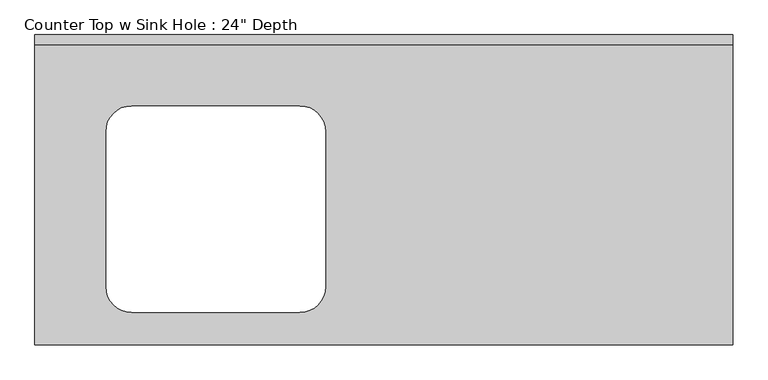
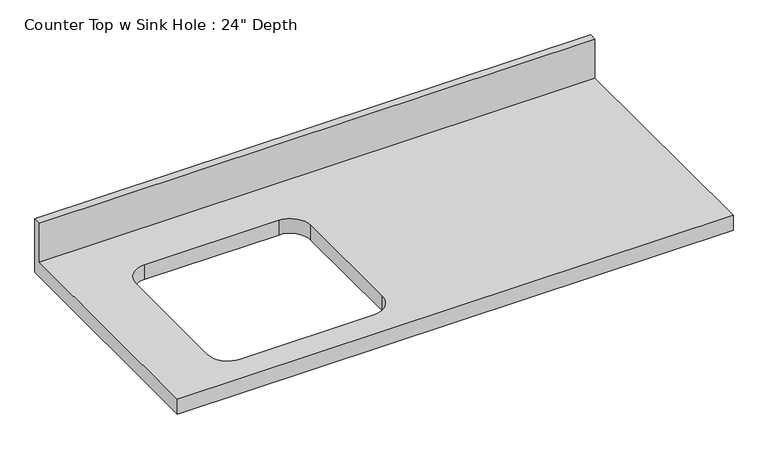
"""IFC4 building model written with IfcOpenShell, lengths in millimetres: furniture geometry."""

from ifc_helpers import new_model, si_unit, frame, origin, place, context, project, spatial, polyline, circle_curve, source, transform, mapped, element, save
from ifc_brep_helpers import plane_surface, revolved_surface, advanced_brep


def furniture_95afb093(model_context):
    return source(origin(), model_context, "Body", "AdvancedBrep", [
        advanced_brep(
        [(-1200.4622951, -609.6, 914.4), (171.1377049, -609.6, 914.4), (171.1377049, -19.05, 914.4), (-1200.4622951, -19.05, 914.4), (-1009.9622951, -139.7, 914.4), (-679.7622951, -139.7, 914.4), (-628.9622951, -190.5, 914.4), (-628.9622951, -495.3, 914.4), (-679.7622951, -546.1, 914.4), (-1009.9622951, -546.1, 914.4), (-1060.7622951, -495.3, 914.4), (-1060.7622951, -190.5, 914.4), (171.1377049, 0.0, 876.3), (171.1377049, -609.6, 876.3), (-1200.4622951, -609.6, 876.3), (-1200.4622951, 0.0, 876.3), (-679.7622951, -139.7, 876.3), (-1009.9622951, -139.7, 876.3), (-1060.7622951, -190.5, 876.3), (-1060.7622951, -495.3, 876.3), (-1009.9622951, -546.1, 876.3), (-679.7622951, -546.1, 876.3), (-628.9622951, -495.3, 876.3), (-628.9622951, -190.5, 876.3), (-1200.4622951, 0.0, 1016.0), (171.1377049, 0.0, 1016.0), (-1200.4622951, -19.05, 1016.0), (171.1377049, -19.05, 1016.0)],
        [
            (0, 1),
            (1, 2),
            (2, 3),
            (3, 0),
            (4, 5),
            (5, 6, circle_curve(frame((-679.7622951, -190.5, 914.4), z_axis=(0.0, 0.0, -1.0), x_axis=(1.0, 0.0, 0.0)), 50.8)),
            (6, 7),
            (7, 8, circle_curve(frame((-679.7622951, -495.3, 914.4), z_axis=(0.0, 0.0, -1.0), x_axis=(1.0, 0.0, 0.0)), 50.8)),
            (8, 9),
            (9, 10, circle_curve(frame((-1009.9622951, -495.3, 914.4), z_axis=(0.0, 0.0, -1.0), x_axis=(1.0, 0.0, 0.0)), 50.8)),
            (10, 11),
            (11, 4, circle_curve(frame((-1009.9622951, -190.5, 914.4), z_axis=(0.0, 0.0, -1.0), x_axis=(1.0, 0.0, 0.0)), 50.8)),
            (12, 13),
            (13, 14),
            (14, 15),
            (15, 12),
            (16, 17),
            (17, 18, circle_curve(frame((-1009.9622951, -190.5, 876.3), z_axis=(0.0, 0.0, 1.0), x_axis=(1.0, 0.0, 0.0)), 50.8)),
            (18, 19),
            (19, 20, circle_curve(frame((-1009.9622951, -495.3, 876.3), z_axis=(0.0, 0.0, 1.0), x_axis=(1.0, 0.0, 0.0)), 50.8)),
            (20, 21),
            (21, 22, circle_curve(frame((-679.7622951, -495.3, 876.3), z_axis=(0.0, 0.0, 1.0), x_axis=(1.0, 0.0, 0.0)), 50.8)),
            (22, 23),
            (23, 16, circle_curve(frame((-679.7622951, -190.5, 876.3), z_axis=(0.0, 0.0, 1.0), x_axis=(1.0, 0.0, 0.0)), 50.8)),
            (15, 24),
            (24, 25),
            (25, 12),
            (14, 0),
            (3, 26),
            (26, 24),
            (13, 1),
            (25, 27),
            (27, 2),
            (4, 17),
            (16, 5),
            (11, 18),
            (10, 19),
            (9, 20),
            (8, 21),
            (7, 22),
            (6, 23),
            (26, 27),
        ],
        [
            plane_surface(frame((-1200.4622951, 0.0, 914.4), z_axis=(0.0, 0.0, 1.0), x_axis=(-1.0, 0.0, 0.0))),
            plane_surface(frame((-1200.4622951, 0.0, 876.3), z_axis=(0.0, 0.0, -1.0), x_axis=(1.0, 0.0, 0.0))),
            plane_surface(frame((171.1377049, 0.0, 914.4), z_axis=(0.0, 1.0, 0.0), x_axis=(0.0, 0.0, -1.0))),
            plane_surface(frame((-1200.4622951, 0.0, 914.4), z_axis=(-1.0, 0.0, 0.0), x_axis=(0.0, 0.0, -1.0))),
            plane_surface(frame((-1200.4622951, -609.6, 914.4), z_axis=(0.0, -1.0, 0.0), x_axis=(0.0, 0.0, -1.0))),
            plane_surface(frame((171.1377049, -609.6, 914.4), z_axis=(1.0, 0.0, 0.0), x_axis=(0.0, 0.0, -1.0))),
            plane_surface(frame((-679.7622951, -139.7, 914.4), z_axis=(0.0, -1.0, 0.0), x_axis=(0.0, 0.0, -1.0))),
            revolved_surface(polyline([(-959.1622951, -190.5, 914.4), (-959.1622951, -190.5, 876.3)]), (-1009.9622951, -190.5, 876.3), (0.0, 0.0, 1.0)),
            plane_surface(frame((-1060.7622951, -190.5, 914.4), z_axis=(1.0, 0.0, 0.0), x_axis=(0.0, 0.0, -1.0))),
            revolved_surface(polyline([(-959.1622951, -495.3, 914.4), (-959.1622951, -495.3, 876.3)]), (-1009.9622951, -495.3, 876.3), (0.0, 0.0, 1.0)),
            plane_surface(frame((-1009.9622951, -546.1, 914.4), z_axis=(0.0, 1.0, 0.0), x_axis=(0.0, 0.0, -1.0))),
            revolved_surface(polyline([(-628.9622951, -495.3, 914.4), (-628.9622951, -495.3, 876.3)]), (-679.7622951, -495.3, 876.3), (0.0, 0.0, 1.0)),
            plane_surface(frame((-628.9622951, -495.3, 914.4), z_axis=(-1.0, 0.0, 0.0), x_axis=(0.0, 0.0, -1.0))),
            revolved_surface(polyline([(-628.9622951, -190.5, 914.4), (-628.9622951, -190.5, 876.3)]), (-679.7622951, -190.5, 876.3), (0.0, 0.0, 1.0)),
            plane_surface(frame((-1200.4622951, 0.0, 1016.0), z_axis=(0.0, 0.0, 1.0), x_axis=(0.0, -1.0, 0.0))),
            plane_surface(frame((-1200.4622951, -19.05, 1016.0), z_axis=(0.0, -1.0, 0.0), x_axis=(0.0, 0.0, -1.0))),
        ],
        [
            (0, [[1, 2, 3, 4], [5, 6, 7, 8, 9, 10, 11, 12]]),
            (1, [[13, 14, 15, 16], [17, 18, 19, 20, 21, 22, 23, 24]]),
            (2, [[-16, 25, 26, 27]]),
            (3, [[-15, 28, -4, 29, 30, -25]]),
            (4, [[-1, -28, -14, 31]]),
            (5, [[-13, -27, 32, 33, -2, -31]]),
            (6, [[34, -17, 35, -5]]),
            (7, [[-34, -12, 36, -18]]),
            (8, [[-36, -11, 37, -19]]),
            (9, [[-37, -10, 38, -20]]),
            (10, [[-38, -9, 39, -21]]),
            (11, [[-39, -8, 40, -22]]),
            (12, [[-40, -7, 41, -23]]),
            (13, [[-35, -24, -41, -6]]),
            (14, [[-30, 42, -32, -26]]),
            (15, [[-42, -29, -3, -33]]),
        ],
    ),
    ])


if __name__ == "__main__":
    model = new_model("IFC4")
    model_context = context("Model", 3, world=origin())
    ifc_project = project(units=[si_unit("LENGTHUNIT", "METRE", prefix="MILLI")], contexts=[model_context])
    site = spatial("IfcSite", under=ifc_project)
    building = spatial("IfcBuilding", under=site)
    placement = place(None, origin())
    furniture_shape = furniture_95afb093(model_context)
    element("IfcFurniture", 1, ObjectType="Counter Top w Sink Hole : 24\" Depth", at=placement, inside=building, context=model_context, shape_type="MappedRepresentation", body=[
        mapped(furniture_shape, transform((0.0, 0.0, 0.0), x_axis=(1.0, 0.0, 0.0), y_axis=(0.0, 1.0, 0.0), z_axis=(0.0, 0.0, 1.0))),
    ])
    save(model, "model.ifc")

# Revit data of these elements
# Type "Counter Top w Sink Hole : 24\" Depth"
#   Assembly Code = "C1030400"
#   Counter Thickness = 0' - 1 1/2"
#   Depth [instance default] = 2' - 1"
#   Height = 3' - 0"
#   Length [instance default] = 8' - 0"
#   Sink Location [instance default] = 2' - 0"
#   Sink Location To Wall [instance default] = 0' - 6"
#   Sink Opening Depth [instance default] = 1' - 3"
#   Sink Opening Width [instance default] = 2' - 3"
#   Counter Top Material = none
#   Default Elevation = 0
# Element 1 (IfcFurniture, "Counter Top w Sink Hole : 24\" Depth")
#   Depth = 2' - 0"
#   Length = 4' - 6"
#   Sink Location = 1' - 2"
#   Sink Opening Width = 1' - 4"
#   Materials on its faces: "Counter Top"
# Materials
#   "Counter Top": class "Wood", colour RGB 226 177 128, transparency 0
